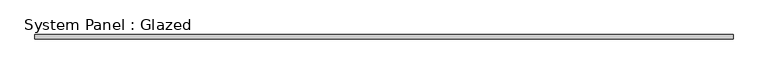
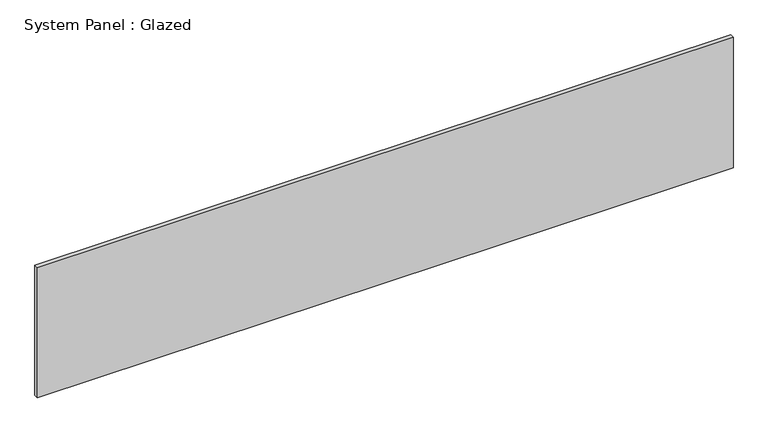
"""IFC4 building model written with IfcOpenShell, lengths in millimetres: plate geometry, System Panel : Glazed."""

from ifc_helpers import new_model, si_unit, origin, origin_with_axes, place, context, project, spatial, polyline, outline, extrude, source, transform, mapped, element, save


def system_panel_glazed_7aae5990(model_context):
    return source(origin(), model_context, "Body", "SweptSolid", [
        extrude(outline(polyline([(2032.0, 19.05), (-2032.0, 19.05), (-2032.0, 44.45), (2032.0, 44.45), (2032.0, 19.05)])), origin_with_axes(), (0.0, 0.0, 1.0), 804.1657953),
    ])


if __name__ == "__main__":
    model = new_model("IFC4")
    model_context = context("Model", 3, world=origin())
    ifc_project = project(units=[si_unit("LENGTHUNIT", "METRE", prefix="MILLI")], contexts=[model_context])
    site = spatial("IfcSite", under=ifc_project)
    building = spatial("IfcBuilding", under=site)
    placement = place(None, origin())
    system_panel_glazed_shape = system_panel_glazed_7aae5990(model_context)
    element("IfcPlate", 1, ObjectType="System Panel : Glazed", at=placement, inside=building, context=model_context, shape_type="MappedRepresentation", body=[
        mapped(system_panel_glazed_shape, transform((0.0, 0.0, 0.0), x_axis=(1.0, 0.0, 0.0), y_axis=(0.0, 1.0, 0.0), z_axis=(0.0, 0.0, 1.0))),
    ])
    save(model, "model.ifc")

# Revit data of these elements
# Type "System Panel : Glazed"
#   Construction Type Id = "GSP4R"
#   Analytic Construction = "1/8 in Pilkington single glazing"
#   Visual Light Transmittance = 0.9
#   Solar Heat Gain Coefficient = 0.86
#   Heat Transfer Coefficient (U) = 1.18115 BTU/(h·ft²·°F)
#   Define Thermal Properties by = 1
# Element 1 (IfcPlate, "System Panel : Glazed")
#   Materials on its faces: "Glass"
# Materials
#   "Glass": class "Glass", colour RGB 0 128 192, transparency 0.75, Description = "Soda Lime Glass", Cost = 0
